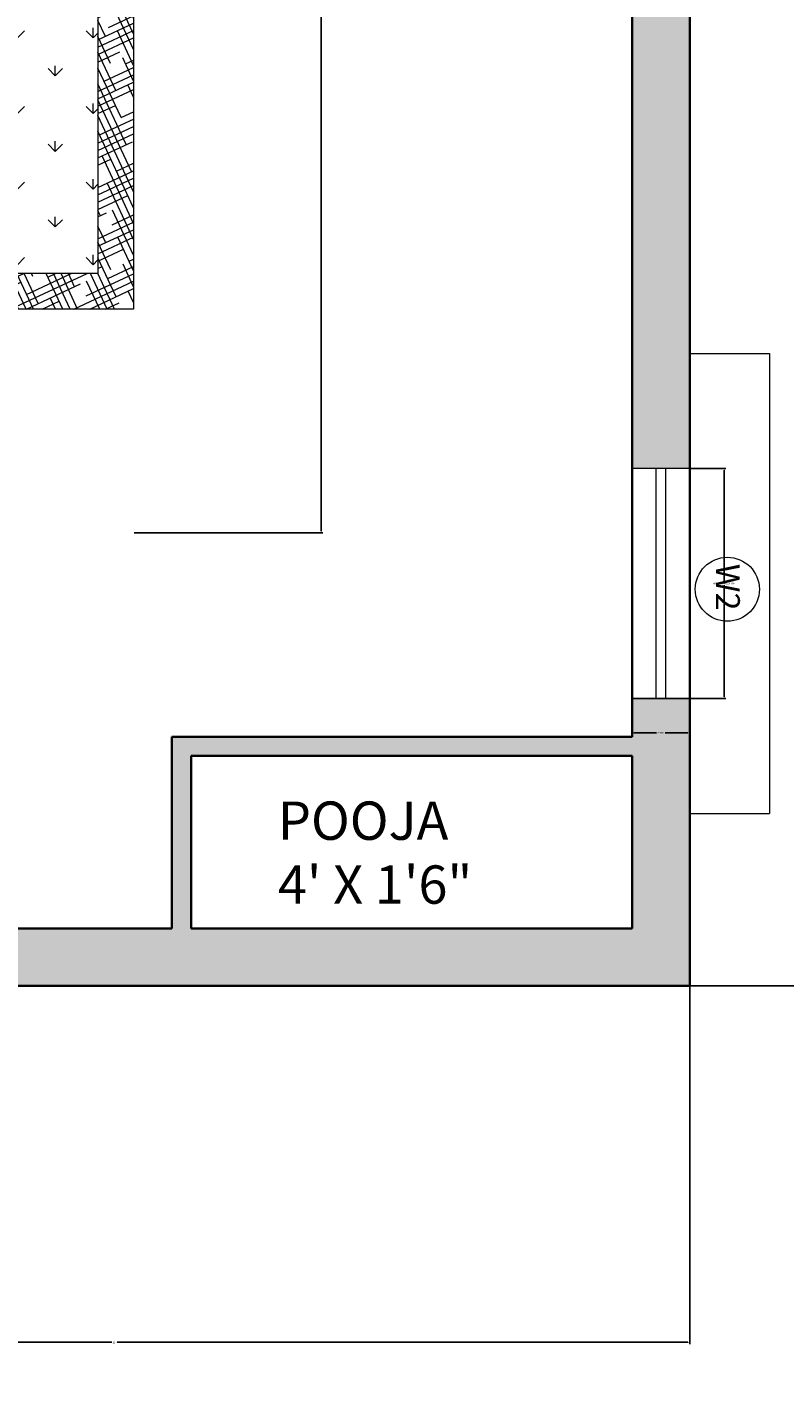
# Model space of a CAD drawing. Units: inches. Extents: x 2701 to 6846, y 811 to 2447.
# Tile 5 of 20: x 3023 to 3102, y 989 to 1130. Entities that reach past the tile are written whole.
import ezdxf

# ---------------------------------------------------------------- set-up
doc = ezdxf.new("R2010")
doc.units = ezdxf.units.IN
for name, color, linetype, lineweight in [('A-ANNO-DIMS', 2, 'Continuous', 18), ('A-ANNO-IDEN', 7, 'Continuous', 13), ('A-AREA-IDEN', 7, 'Continuous', 18), ('A-FURN', 8, 'Continuous', 13), ('A-GLAZ', 4, 'Continuous', 18), ('A-WALL', 7, 'Continuous', 35)]:
    doc.layers.add(name, color=color, linetype=linetype, lineweight=lineweight)
doc.layers.add('A-WALL-PATT', color=18, linetype='Continuous', lineweight=13, true_color=0x000000)
doc.styles.get("Standard").update_dxf_attribs({"font": 'arial.ttf'})
doc.dimstyles.get("Standard").update_dxf_attribs({"dimtxt": 0.18, "dimasz": 0.18, "dimexe": 0.18, "dimexo": 0.0625, "dimgap": 0.09, "dimtad": 0, "dimtih": 1, "dimtoh": 1, "dimdec": 4, "dimzin": 0, "dimdsep": 46, "dimtxsty": 'Standard', "dimcen": 0.09, "dimadec": 0, "dimazin": 0, "dimtfac": 1, "dimtdec": 4, "dimtofl": 0, "dimtmove": 0, "dimatfit": 3, "dimfxl": 1, "dimtolj": 1, "dimtzin": 0, "dimarcsym": 0})

# ---------------------------------------------------------------- blocks, each defined once
blk = doc.blocks.new('A$C0782773B')
for p, q in [((1027.2, 2344.2), (2528, 2344.2)), ((1508.8, 2344.2), (1508.8, 1489.7)), ((2046.4, 2344.2), (2046.4, 1489.7)), ((3223.5, 2286.1), (2888.9, 2183.3)), ((3429.1, 1617), (3223.5, 2286.1)), ((3197, 2236.1), (2938.9, 2156.8)), ((3379.1, 1643.5), (3197, 2236.1)), ((909.6, 2226.6), (909.6, 2215.4)), ((2645.6, 2226.6), (2645.6, 2215.4)), ((859.2, 2176.2), (859.2, 1545.7)), ((2696, 2176.2), (2696, 1545.7)), ((2888.9, 2183.3), (3094.6, 1514.2)), ((2938.9, 2156.8), (3121.1, 1564.2)), ((971.2, 2111.9), (971.2, 1657.7)), ((1027.2, 2097.8), (2528, 2097.8)), ((2584, 2111.9), (2584, 1657.7)), ((971.2, 2013.8), (2584, 2013.8)), ((622.9, 1770.7), (643.4, 1780.2)), ((622.9, 1750), (687.8, 1780.2)), ((622.9, 1729.3), (732.1, 1780.2)), ((622.9, 1380.2), (622.9, 1780.2)), ((622.9, 1780.2), (859.2, 1780.2)), ((627.3, 1710.7), (776.5, 1780.2)), ((636.3, 1780.2), (637.5, 1777.5)), ((657, 1780.2), (686.2, 1717.5)), ((677.6, 1780.2), (724.3, 1680.2)), ((698.3, 1780.2), (745, 1680.2)), ((703.2, 1725.4), (820.8, 1780.2)), ((719, 1780.2), (765.7, 1680.2)), ((754.2, 1749.2), (786.3, 1680.2)), ((779.1, 1740.1), (859.2, 1777.4)), ((781.1, 1780.2), (788.2, 1765)), ((801.8, 1780.2), (836.9, 1705)), ((822.5, 1780.2), (859.2, 1701.5)), ((843.2, 1780.2), (859.2, 1745.8)), ((855, 1754.8), (859.2, 1756.8)), ((2696, 1682.3), (2906.1, 1780.2)), ((2696, 1780.2), (3012.8, 1780.2)), ((2696, 1703), (2835, 1767.8)), ((2696, 1755.4), (2731, 1680.2)), ((2696, 1723.7), (2759.1, 1753.1)), ((2717.2, 1754.3), (2751.7, 1680.2)), ((2736, 1680.2), (2950.4, 1780.2)), ((2746.5, 1780.2), (2751.2, 1770.1)), ((2767.2, 1780.2), (2799.9, 1710.1)), ((2787.9, 1780.2), (2834.5, 1680.2)), ((2790.8, 1685.1), (2994.8, 1780.2)), ((2808.5, 1780.2), (2855.2, 1680.2)), ((2829.2, 1780.2), (2875.9, 1680.2)), ((2866.7, 1699.8), (3016.1, 1769.5)), ((2891.3, 1780.2), (2901.9, 1757.6)), ((2912, 1780.2), (2950.5, 1697.6)), ((2932.7, 1780.2), (2999.2, 1637.5)), ((2942.6, 1714.5), (3021.7, 1751.4)), ((2953.4, 1780.2), (3039.7, 1595.1)), ((2974, 1780.2), (3039.7, 1639.5)), ((622.9, 1720.3), (722.9, 1505.8)), ((739.5, 1680.2), (795, 1706.1)), ((783.9, 1680.2), (859.2, 1715.4)), ((2696, 1711), (2710.4, 1680.2)), ((2867.9, 1741.8), (2896.6, 1680.2)), ((3018.5, 1729.2), (3027.2, 1733.3)), ((3018.5, 1729.2), (3039.7, 1683.9)), ((622.9, 1646.6), (719.1, 1691.4)), ((622.9, 1667.2), (643.2, 1676.7)), ((622.9, 1675.9), (681.6, 1549.8)), ((622.9, 1625.9), (722.9, 1672.5)), ((652.2, 1701.6), (722.9, 1550.2)), ((722.9, 1340.4), (722.9, 1680.2)), ((722.9, 1680.2), (859.2, 1680.2)), ((802.9, 1689.1), (807, 1680.2)), ((828.2, 1680.2), (859.2, 1694.7)), ((2696, 1680.2), (2939.7, 1680.2)), ((2765.9, 1694.2), (2772.4, 1680.2)), ((2916.6, 1681.7), (2917.2, 1680.2)), ((2939.7, 1651.1), (3034.4, 1695.3)), ((2939.7, 1671.8), (2958.5, 1680.6)), ((2939.7, 1680.2), (2939.7, 1461.7)), ((2939.7, 1630.4), (3039.7, 1677.1)), ((3039.7, 1692.8), (3039.7, 1461.7)), ((622.9, 1605.2), (722.9, 1651.8)), ((622.9, 1631.5), (633, 1609.9)), ((674.9, 1608.7), (722.9, 1631.1)), ((700.9, 1641.6), (722.9, 1594.5)), ((2939.7, 1609.7), (3039.7, 1656.4)), ((2939.7, 1632.1), (3019.1, 1461.7)), ((2990.2, 1612.6), (3039.7, 1635.7)), ((3121.1, 1564.2), (3379.1, 1643.5)), ((747.4, 1598.5), (767.3, 1618.4)), ((747.4, 1598.5), (775.6, 1598.5)), ((747.4, 1598.5), (767.3, 1578.6)), ((2868.8, 1598.5), (2888.7, 1618.4)), ((2868.8, 1598.5), (2896.9, 1598.5)), ((2868.8, 1598.5), (2888.7, 1578.6)), ((2965.3, 1621.7), (3039.7, 1462)), ((3094.6, 1514.2), (3429.1, 1617)), ((622.9, 1543.1), (690.7, 1574.7)), ((622.9, 1522.4), (722.9, 1569.1)), ((2939.7, 1587.7), (2994.7, 1469.9)), ((2939.7, 1547.7), (3006, 1578.6)), ((2939.7, 1527), (3039.7, 1573.6)), ((3013.9, 1561.6), (3039.7, 1506.4)), ((622.9, 1501.7), (722.9, 1548.4)), ((622.9, 1542.8), (715.9, 1343.2)), ((646.5, 1492.1), (722.9, 1527.7)), ((647.7, 1534), (722.9, 1372.7)), ((2939.7, 1506.3), (3039.7, 1552.9)), ((2939.7, 1543.4), (2946, 1529.9)), ((2961.8, 1495.9), (3039.7, 1532.2)), ((622.9, 1498.4), (677.1, 1382.2)), ((722.4, 1506.8), (722.9, 1507)), ((853.5, 1492.5), (871.6, 1510.6)), ((853.5, 1492.5), (881.6, 1492.5)), ((853.5, 1492.5), (873.4, 1472.6)), ((915.2, 1489.7), (2640, 1489.7)), ((1068.4, 1489.7), (1085.5, 1472.6)), ((1280.5, 1489.7), (1297.7, 1472.6)), ((1492.7, 1489.7), (1509.8, 1472.6)), ((1704.8, 1489.7), (1721.9, 1472.6)), ((1916.9, 1489.7), (1934.1, 1472.6)), ((2129.1, 1489.7), (2146.2, 1472.6)), ((2341.2, 1489.7), (2358.3, 1472.6)), ((2553.3, 1489.7), (2570.5, 1472.6)), ((2762.7, 1492.5), (2782.6, 1512.3)), ((2762.7, 1492.5), (2790.8, 1492.5)), ((2762.7, 1492.5), (2782.6, 1472.6)), ((3037.7, 1510.6), (3039.7, 1511.5)), ((395.3, 1470.7), (915.7, 1263.8)), ((622.9, 1419), (722.9, 1465.6)), ((622.9, 1439.7), (662.4, 1458.1)), ((622.9, 1454.1), (628.4, 1442.2)), ((622.9, 1398.3), (722.9, 1444.9)), ((696.4, 1473.9), (722.9, 1417.1)), ((3326.7, 1461.7), (2766.7, 1461.7)), ((2977.2, 1461.7), (2977.7, 1461.9)), ((3021.6, 1461.7), (3039.7, 1470.2)), ((625.9, 1379), (722.9, 1424.2)), ((694.1, 1390.1), (722.9, 1403.5)), ((747.4, 1386.4), (767.3, 1406.3)), ((959.6, 1386.4), (979.5, 1406.3)), ((1171.7, 1386.4), (1191.6, 1406.3)), ((1383.8, 1386.4), (1403.7, 1406.3)), ((1596, 1386.4), (1615.9, 1406.3)), ((1808.1, 1386.4), (1828, 1406.3)), ((2020.2, 1386.4), (2040.1, 1406.3)), ((2232.4, 1386.4), (2252.3, 1406.3)), ((2444.5, 1386.4), (2464.4, 1406.3)), ((2656.6, 1386.4), (2676.5, 1406.3)), ((2710.7, 1349.7), (2710.7, 1405.7)), ((747.4, 1386.4), (775.6, 1386.4)), ((747.4, 1386.4), (767.3, 1366.5)), ((959.6, 1386.4), (987.7, 1386.4)), ((959.6, 1386.4), (979.5, 1366.5)), ((1171.7, 1386.4), (1199.8, 1386.4)), ((1171.7, 1386.4), (1191.6, 1366.5)), ((1383.8, 1386.4), (1412, 1386.4)), ((1383.8, 1386.4), (1403.7, 1366.5)), ((1596, 1386.4), (1624.1, 1386.4)), ((1596, 1386.4), (1615.9, 1366.5)), ((1808.1, 1386.4), (1836.2, 1386.4)), ((1808.1, 1386.4), (1828, 1366.5)), ((2020.2, 1386.4), (2048.4, 1386.4)), ((2020.2, 1386.4), (2040.1, 1366.5)), ((2232.4, 1386.4), (2260.5, 1386.4)), ((2232.4, 1386.4), (2252.3, 1366.5)), ((2444.5, 1386.4), (2472.6, 1386.4)), ((2444.5, 1386.4), (2464.4, 1366.5)), ((2656.6, 1386.4), (2684.8, 1386.4)), ((2656.6, 1386.4), (2676.5, 1366.5)), ((413.6, 1342.9), (770.2, 1201.1)), ((697.7, 1350.4), (709.9, 1356.1)), ((721.7, 1340.9), (722.9, 1341.5)), ((2710.7, 1349.7), (2710.7, 733.3)), ((3262.5, 1349.7), (2878.7, 1349.7)), ((3164.3, 1349.7), (3164.3, 789.3)), ((11.5, 960), (148, 1303.4)), ((297.8, 785.9), (504.9, 1306.6)), ((859.4, 1286.2), (873.4, 1300.2)), ((1065.6, 1280.3), (1085.5, 1300.2)), ((1277.8, 1280.3), (1297.7, 1300.2)), ((1489.9, 1280.3), (1509.8, 1300.2)), ((1702, 1280.3), (1721.9, 1300.2)), ((1914.2, 1280.3), (1934.1, 1300.2)), ((2126.3, 1280.3), (2146.2, 1300.2)), ((2338.4, 1280.3), (2358.3, 1300.2)), ((2550.6, 1280.3), (2570.5, 1300.2)), ((3248.3, 1293.7), (3248.3, 924.1)), ((3494.7, 1293.7), (3494.7, 924.1)), ((874.1, 1280.3), (881.6, 1280.3)), ((1065.6, 1280.3), (1093.8, 1280.3)), ((1065.6, 1280.3), (1085.5, 1260.4)), ((1277.8, 1280.3), (1305.9, 1280.3)), ((1277.8, 1280.3), (1297.7, 1260.4)), ((1489.9, 1280.3), (1518, 1280.3)), ((1489.9, 1280.3), (1509.8, 1260.4)), ((1702, 1280.3), (1730.2, 1280.3)), ((1702, 1280.3), (1721.9, 1260.4)), ((1914.2, 1280.3), (1942.3, 1280.3)), ((1914.2, 1280.3), (1934.1, 1260.4)), ((2126.3, 1280.3), (2154.4, 1280.3)), ((2126.3, 1280.3), (2146.2, 1260.4)), ((2338.4, 1280.3), (2366.6, 1280.3)), ((2338.4, 1280.3), (2358.3, 1260.4)), ((2550.6, 1280.3), (2578.7, 1280.3)), ((2550.6, 1280.3), (2570.5, 1260.4)), ((240.4, 868.9), (377, 1212.4)), ((719.3, 618.3), (947, 1191)), ((959.6, 1174.3), (979.5, 1194.1)), ((1171.7, 1174.3), (1191.6, 1194.1)), ((1383.8, 1174.3), (1403.7, 1194.1)), ((1596, 1174.3), (1615.9, 1194.1)), ((1808.1, 1174.3), (1828, 1194.1)), ((2020.2, 1174.3), (2040.1, 1194.1)), ((2232.4, 1174.3), (2252.3, 1194.1)), ((2444.5, 1174.3), (2464.4, 1194.1)), ((2656.6, 1174.3), (2676.5, 1194.1)), ((959.6, 1174.3), (987.7, 1174.3)), ((959.6, 1174.3), (979.5, 1154.4)), ((1171.7, 1174.3), (1199.8, 1174.3)), ((1171.7, 1174.3), (1191.6, 1154.4)), ((1383.8, 1174.3), (1412, 1174.3)), ((1383.8, 1174.3), (1403.7, 1154.4)), ((1596, 1174.3), (1624.1, 1174.3)), ((1596, 1174.3), (1615.9, 1154.4)), ((1808.1, 1174.3), (1836.2, 1174.3)), ((1808.1, 1174.3), (1828, 1154.4)), ((2020.2, 1174.3), (2048.4, 1174.3)), ((2020.2, 1174.3), (2040.1, 1154.4)), ((2232.4, 1174.3), (2260.5, 1174.3)), ((2232.4, 1174.3), (2252.3, 1154.4)), ((2444.5, 1174.3), (2472.6, 1174.3)), ((2444.5, 1174.3), (2464.4, 1154.4)), ((2656.6, 1174.3), (2684.8, 1174.3)), ((2656.6, 1174.3), (2676.5, 1154.4)), ((1358.2, 528.2), (1358.2, 1102.6)), ((1358.2, 1102.6), (2266.7, 1102.6)), ((2266.7, 1102.6), (2266.7, 528.2)), ((1065.6, 1068.2), (1085.5, 1088.1)), ((1065.6, 1068.2), (1093.8, 1068.2)), ((1065.6, 1068.2), (1085.5, 1048.3)), ((1277.8, 1068.2), (1297.7, 1088.1)), ((1277.8, 1068.2), (1305.9, 1068.2)), ((1277.8, 1068.2), (1297.7, 1048.3)), ((2338.4, 1068.2), (2358.3, 1088.1)), ((2338.4, 1068.2), (2366.6, 1068.2)), ((2338.4, 1068.2), (2358.3, 1048.3)), ((2550.6, 1068.2), (2570.5, 1088.1)), ((2550.6, 1068.2), (2578.7, 1068.2)), ((2550.6, 1068.2), (2570.5, 1048.3)), ((1408.2, 578.2), (1408.2, 1052.6)), ((1408.2, 1052.6), (2216.7, 1052.6)), ((1408.2, 1031.9), (1644.7, 847.1)), ((1437.7, 1052.6), (1999.3, 613.9)), ((1510.8, 1052.6), (2118.1, 578.2)), ((1674, 1052.6), (1887.9, 885.5)), ((1681.3, 1052.6), (2216.7, 634.3)), ((1738, 1027.4), (2092.6, 750.4)), ((1837.3, 1052.6), (1926.1, 983.2)), ((1925, 1052.6), (2216.7, 824.7)), ((2000.5, 1052.6), (2216.7, 883.7)), ((2029.7, 1052.6), (2097.2, 999.9)), ((2163.7, 1052.6), (2215.4, 1012.3)), ((2168.6, 1052.6), (2216.7, 1015)), ((2216.7, 1052.6), (2216.7, 578.2)), ((1408.2, 1005.3), (1598.7, 856.4)), ((959.6, 962.1), (979.5, 982)), ((959.6, 962.1), (987.7, 962.1)), ((959.6, 962.1), (979.5, 942.2)), ((1171.7, 962.1), (1191.6, 982)), ((1171.7, 962.1), (1199.8, 962.1)), ((1171.7, 962.1), (1191.6, 942.2)), ((2136.2, 969.5), (2216.7, 906.5)), ((2444.5, 962.1), (2464.4, 982)), ((2444.5, 962.1), (2472.6, 962.1)), ((2444.5, 962.1), (2464.4, 942.2)), ((2656.6, 962.1), (2676.5, 982)), ((2656.6, 962.1), (2684.8, 962.1)), ((2656.6, 962.1), (2676.5, 942.2)), ((853.5, 856.1), (873.4, 876)), ((1065.6, 856.1), (1085.5, 876)), ((1277.8, 856.1), (1297.7, 876)), ((1408.2, 885.3), (1646.9, 698.8)), ((1408.2, 877.7), (1560.4, 758.8)), ((2338.4, 856.1), (2358.3, 876)), ((2550.6, 856.1), (2570.5, 876)), ((853.5, 856.1), (881.6, 856.1)), ((853.5, 856.1), (873.4, 836.2)), ((1065.6, 856.1), (1093.8, 856.1)), ((1065.6, 856.1), (1085.5, 836.2)), ((1277.8, 856.1), (1305.9, 856.1)), ((1277.8, 856.1), (1297.7, 836.2)), ((2091.6, 853.9), (2216.7, 756.2)), ((2338.4, 856.1), (2366.6, 856.1)), ((2338.4, 856.1), (2358.3, 836.2)), ((2550.6, 856.1), (2578.7, 856.1)), ((2550.6, 856.1), (2570.5, 836.2)), ((206.6, 822.1), (563.2, 680.3)), ((959.6, 750), (979.5, 769.9)), ((1171.7, 750), (1191.6, 769.9)), ((1408.2, 778.7), (1640.1, 597.6)), ((1733.4, 777.9), (1989, 578.2)), ((2006.1, 793.2), (2216.7, 628.6)), ((2444.5, 750), (2464.4, 769.9)), ((2656.6, 750), (2676.5, 769.9)), ((3262.5, 789.3), (2878.7, 789.3)), ((105.5, 741.8), (625.9, 534.9)), ((764.8, 732.7), (767.3, 730.1)), ((771.7, 750), (775.6, 750)), ((959.6, 750), (987.7, 750)), ((959.6, 750), (979.5, 730.1)), ((1171.7, 750), (1199.8, 750)), ((1171.7, 750), (1191.6, 730.1)), ((1408.2, 750.2), (1628.4, 578.2)), ((1764.2, 727.1), (1954.8, 578.2)), ((2131.6, 719.9), (2216.7, 653.4)), ((2444.5, 750), (2472.6, 750)), ((2444.5, 750), (2464.4, 730.1)), ((2656.6, 750), (2684.8, 750)), ((2656.6, 750), (2676.5, 730.1)), ((853.5, 643.9), (873.4, 663.8)), ((1065.6, 643.9), (1085.5, 663.8)), ((1277.8, 643.9), (1297.7, 663.8)), ((1678.6, 666.4), (1791.6, 578.2)), ((2338.4, 643.9), (2358.3, 663.8)), ((2550.6, 643.9), (2570.5, 663.8)), ((2762.7, 643.9), (2782.6, 663.8)), ((3326.7, 677.3), (2766.7, 677.3)), ((2939.7, 658.1), (2981, 677.3)), ((2939.7, 637.4), (3025.4, 677.3)), ((2939.7, 677.3), (2939.7, 567.7)), ((2939.7, 616.7), (3039.7, 663.3)), ((2950.4, 677.3), (2971.8, 631.6)), ((2971.1, 677.3), (3020.4, 571.6)), ((2991.8, 677.3), (3039.7, 574.7)), ((3012.5, 677.3), (3039.7, 619.1)), ((3039.7, 677.3), (3039.7, 567.7)), ((719.3, 618.3), (698.6, 566.2)), ((722.9, 100), (722.9, 627.2)), ((853.5, 643.9), (881.6, 643.9)), ((853.5, 643.9), (873.4, 624)), ((1065.6, 643.9), (1093.8, 643.9)), ((1065.6, 643.9), (1085.5, 624)), ((1277.8, 643.9), (1305.9, 643.9)), ((1277.8, 643.9), (1297.7, 624)), ((2338.4, 643.9), (2366.6, 643.9)), ((2338.4, 643.9), (2358.3, 624)), ((2550.6, 643.9), (2578.7, 643.9)), ((2550.6, 643.9), (2570.5, 624)), ((2762.7, 643.9), (2790.8, 643.9)), ((2762.7, 643.9), (2782.6, 624)), ((2939.7, 611.7), (2960.2, 567.7)), ((2962.7, 606.7), (3039.7, 642.6)), ((3038.6, 621.4), (3039.7, 621.9)), ((697.8, 564.3), (722.9, 576)), ((701.9, 574.6), (722.9, 529.8)), ((722.1, 575.7), (722.9, 574.1)), ((2216.7, 578.2), (1408.2, 578.2)), ((1436.7, 600.4), (1465.1, 578.2)), ((1530.9, 599.1), (1557.7, 578.2)), ((2967.7, 567.7), (2978.5, 572.7)), ((3012, 567.7), (3039.7, 580.6)), ((622.9, 508.7), (722.9, 555.3)), ((622.9, 0), (622.9, 536.1)), ((622.9, 488), (722.9, 534.6)), ((622.9, 529.4), (630.9, 533.1)), ((676.8, 539.8), (702.9, 483.9)), ((691.3, 553.2), (722.9, 485.4)), ((747.4, 537.9), (767.3, 557.8)), ((747.4, 537.9), (775.6, 537.9)), ((747.4, 537.9), (767.3, 518)), ((959.6, 537.9), (979.5, 557.8)), ((959.6, 537.9), (987.7, 537.9)), ((959.6, 537.9), (979.5, 518)), ((1171.7, 537.9), (1191.6, 557.8)), ((1171.7, 537.9), (1199.8, 537.9)), ((1171.7, 537.9), (1191.6, 518)), ((2444.5, 537.9), (2464.4, 557.8)), ((2444.5, 537.9), (2472.6, 537.9)), ((2444.5, 537.9), (2464.4, 518)), ((2656.6, 537.9), (2676.5, 557.8)), ((2656.6, 537.9), (2684.8, 537.9)), ((2656.6, 537.9), (2676.5, 518)), ((2868.8, 537.9), (2873.3, 542.4)), ((2868.8, 537.9), (2873.3, 537.9)), ((2868.8, 537.9), (2873.3, 533.3)), ((2873.3, 567.7), (3323.3, 567.7)), ((2873.3, 117.7), (2873.3, 567.7)), ((3323.3, 567.7), (3323.3, 117.7)), ((622.9, 522.4), (722.9, 307.9)), ((694.9, 500.9), (722.9, 513.9)), ((2266.7, 528.2), (1358.2, 528.2)), ((1393.5, 528.2), (1403.7, 518)), ((1605.7, 528.2), (1615.9, 518)), ((1817.8, 528.2), (1828, 518)), ((2029.9, 528.2), (2040.1, 518)), ((2242.1, 528.2), (2252.3, 518)), ((3098.3, 156.5), (3098.3, 526.4)), ((622.9, 478), (698.3, 316.3)), ((622.9, 425.9), (710.8, 466.9)), ((668.9, 468.1), (722.9, 352.3)), ((622.9, 446.6), (634.9, 452.2)), ((622.9, 405.3), (722.9, 451.9)), ((622.9, 433.6), (649.6, 376.3)), ((622.9, 384.6), (722.9, 431.2)), ((853.5, 431.8), (873.4, 451.7)), ((853.5, 431.8), (881.6, 431.8)), ((853.5, 431.8), (873.4, 411.9)), ((1065.6, 431.8), (1085.5, 451.7)), ((1065.6, 431.8), (1093.8, 431.8)), ((1065.6, 431.8), (1085.5, 411.9)), ((1277.8, 431.8), (1297.7, 451.7)), ((1277.8, 431.8), (1305.9, 431.8)), ((1277.8, 431.8), (1297.7, 411.9)), ((1489.9, 431.8), (1509.8, 451.7)), ((1489.9, 431.8), (1518, 431.8)), ((1489.9, 431.8), (1509.8, 411.9)), ((1702, 431.8), (1721.9, 451.7)), ((1702, 431.8), (1730.2, 431.8)), ((1702, 431.8), (1721.9, 411.9)), ((1914.2, 431.8), (1934.1, 451.7)), ((1914.2, 431.8), (1942.3, 431.8)), ((1914.2, 431.8), (1934.1, 411.9)), ((2126.3, 431.8), (2146.2, 451.7)), ((2126.3, 431.8), (2154.4, 431.8)), ((2126.3, 431.8), (2146.2, 411.9)), ((2338.4, 431.8), (2358.3, 451.7)), ((2338.4, 431.8), (2366.6, 431.8)), ((2338.4, 431.8), (2358.3, 411.9)), ((2550.6, 431.8), (2570.5, 451.7)), ((2550.6, 431.8), (2578.7, 431.8)), ((2550.6, 431.8), (2570.5, 411.9)), ((2762.7, 431.8), (2782.6, 451.7)), ((2762.7, 431.8), (2790.8, 431.8)), ((2762.7, 431.8), (2782.6, 411.9)), ((666.6, 384.3), (722.9, 410.5)), ((717.6, 408), (722.9, 396.7)), ((622.9, 322.5), (682.4, 350.3)), ((622.9, 301.8), (722.9, 348.4)), ((622.9, 344.9), (722.9, 130.5)), ((747.4, 325.7), (767.3, 345.6)), ((959.6, 325.7), (979.5, 345.6)), ((1171.7, 325.7), (1191.6, 345.6)), ((1383.8, 325.7), (1403.7, 345.6)), ((1596, 325.7), (1615.9, 345.6)), ((1808.1, 325.7), (1828, 345.6)), ((2020.2, 325.7), (2040.1, 345.6)), ((2232.4, 325.7), (2252.3, 345.6)), ((2444.5, 325.7), (2464.4, 345.6)), ((2656.6, 325.7), (2676.5, 345.6)), ((2914.5, 342.7), (3284.1, 342.7)), ((622.9, 281.1), (722.9, 327.8)), ((638.2, 267.6), (722.9, 307.1)), ((747.4, 325.7), (775.6, 325.7)), ((747.4, 325.7), (767.3, 305.8)), ((959.6, 325.7), (987.7, 325.7)), ((959.6, 325.7), (979.5, 305.8)), ((1171.7, 325.7), (1199.8, 325.7)), ((1171.7, 325.7), (1191.6, 305.8)), ((1383.8, 325.7), (1412, 325.7)), ((1383.8, 325.7), (1403.7, 305.8)), ((1596, 325.7), (1624.1, 325.7)), ((1596, 325.7), (1615.9, 305.8)), ((1808.1, 325.7), (1836.2, 325.7)), ((1808.1, 325.7), (1828, 305.8)), ((2020.2, 325.7), (2048.4, 325.7)), ((2020.2, 325.7), (2040.1, 305.8)), ((2232.4, 325.7), (2260.5, 325.7)), ((2232.4, 325.7), (2252.3, 305.8)), ((2444.5, 325.7), (2472.6, 325.7)), ((2444.5, 325.7), (2464.4, 305.8)), ((2656.6, 325.7), (2684.8, 325.7)), ((2656.6, 325.7), (2676.5, 305.8)), ((2868.8, 325.7), (2873.3, 330.3)), ((2868.8, 325.7), (2873.3, 325.7)), ((2868.8, 325.7), (2873.3, 321.2)), ((622.9, 300.5), (693.7, 148.6)), ((664.3, 300.4), (722.9, 174.8)), ((714.1, 282.3), (722.9, 286.4)), ((622.9, 256.2), (645, 208.7)), ((622.9, 198.4), (722.9, 245)), ((622.9, 219.1), (654.1, 233.6)), ((713, 240.4), (722.9, 219.2)), ((853.5, 219.7), (873.4, 239.6)), ((1065.6, 219.7), (1085.5, 239.6)), ((1277.8, 219.7), (1297.7, 239.6)), ((1489.9, 219.7), (1509.8, 239.6)), ((1702, 219.7), (1721.9, 239.6)), ((1914.2, 219.7), (1934.1, 239.6)), ((2126.3, 219.7), (2146.2, 239.6)), ((2338.4, 219.7), (2358.3, 239.6)), ((2550.6, 219.7), (2570.5, 239.6)), ((2762.7, 219.7), (2782.6, 239.6)), ((622.9, 177.7), (722.9, 224.3)), ((622.9, 157), (722.9, 203.6)), ((853.5, 219.7), (881.6, 219.7)), ((853.5, 219.7), (873.4, 199.8)), ((1065.6, 219.7), (1093.8, 219.7)), ((1065.6, 219.7), (1085.5, 199.8)), ((1277.8, 219.7), (1305.9, 219.7)), ((1277.8, 219.7), (1297.7, 199.8)), ((1489.9, 219.7), (1518, 219.7)), ((1489.9, 219.7), (1509.8, 199.8)), ((1702, 219.7), (1730.2, 219.7)), ((1702, 219.7), (1721.9, 199.8)), ((1914.2, 219.7), (1942.3, 219.7)), ((1914.2, 219.7), (1934.1, 199.8)), ((2126.3, 219.7), (2154.4, 219.7)), ((2126.3, 219.7), (2146.2, 199.8)), ((2338.4, 219.7), (2366.6, 219.7)), ((2338.4, 219.7), (2358.3, 199.8)), ((2550.6, 219.7), (2578.7, 219.7)), ((2550.6, 219.7), (2570.5, 199.8)), ((2762.7, 219.7), (2790.8, 219.7)), ((2762.7, 219.7), (2782.6, 199.8)), ((622.9, 167.4), (700.9, 0)), ((685.8, 165.6), (722.9, 182.9)), ((622.9, 94.9), (701.6, 131.7)), ((622.9, 123.1), (680.3, 0)), ((622.9, 74.2), (722.9, 120.9)), ((622.9, 115.6), (625.7, 116.9)), ((659.7, 132.8), (721.6, 0)), ((747.4, 113.6), (767.3, 133.5)), ((959.6, 113.6), (979.5, 133.5)), ((1171.7, 113.6), (1191.6, 133.5)), ((1383.8, 113.6), (1403.7, 133.5)), ((1596, 113.6), (1615.9, 133.5)), ((1808.1, 113.6), (1828, 133.5)), ((2020.2, 113.6), (2040.1, 133.5)), ((2232.4, 113.6), (2252.3, 133.5)), ((2444.5, 113.6), (2464.4, 133.5)), ((2656.6, 113.6), (2676.5, 133.5)), ((2745, 8.7), (2978.7, 117.7)), ((2820.9, 23.4), (3023, 117.7)), ((2868.8, 113.6), (2873.3, 118.1)), ((3323.3, 117.7), (2873.3, 117.7)), ((2939.7, 117.7), (2939.7, 100)), ((2983.9, 117.7), (3006.7, 68.7)), ((3004.5, 117.7), (3039.7, 42.3)), ((3025.2, 117.7), (3039.7, 86.7)), ((3039.7, 117.7), (3039.7, 0)), ((622.9, 53.5), (722.9, 100.2)), ((622.9, 78.7), (640.4, 41)), ((657.4, 49), (766.8, 100)), ((2939.7, 100), (722.9, 100)), ((733.3, 63.7), (811.2, 100)), ((737.1, 100), (742.4, 88.6)), ((747.4, 113.6), (775.6, 113.6)), ((747.4, 113.6), (761, 100)), ((757.8, 100), (791.1, 28.5)), ((778.4, 100), (825.1, 0)), ((799.1, 100), (845.8, 0)), ((809.2, 78.4), (855.6, 100)), ((819.8, 100), (866.5, 0)), ((863, 0), (1052.8, 88.5)), ((881.9, 100), (893, 76.1)), ((885.1, 93.1), (899.9, 100)), ((902.6, 100), (941.7, 16)), ((907.3, 0), (1121.8, 100)), ((923.3, 100), (969.9, 0)), ((943.9, 100), (990.6, 0)), ((951.7, 0), (1166.1, 100)), ((959.6, 113.6), (987.7, 113.6)), ((959.6, 113.6), (973.2, 100)), ((964.6, 100), (1011.3, 0)), ((1008.6, 5.8), (1210.5, 100)), ((1026.7, 100), (1043.7, 63.6)), ((1047.4, 100), (1092.4, 3.5)), ((1068.1, 100), (1114.7, 0)), ((1084.4, 20.5), (1254.9, 100)), ((1088.8, 100), (1135.4, 0)), ((1111.7, 95.3), (1156.1, 0)), ((1160.3, 35.2), (1299.2, 100)), ((1171.5, 100), (1194.3, 51.1)), ((1171.7, 113.6), (1199.8, 113.6)), ((1171.7, 113.6), (1185.3, 100)), ((1192.2, 100), (1238.8, 0)), ((1212.9, 100), (1259.5, 0)), ((1233.6, 100), (1280.2, 0)), ((1236.2, 49.9), (1343.6, 100)), ((1262.3, 82.8), (1300.9, 0)), ((1295.7, 100), (1296.3, 98.6)), ((1312.1, 64.6), (1388, 100)), ((1316.3, 100), (1345, 38.6)), ((1337, 100), (1383.7, 0)), ((1357.7, 100), (1404.3, 0)), ((1378.4, 100), (1425, 0)), ((1383.8, 113.6), (1412, 113.6)), ((1383.8, 113.6), (1397.4, 100)), ((1388, 79.3), (1432.3, 100)), ((1439.7, 0), (1631.6, 89.5)), ((1440.5, 100), (1446.9, 86.1)), ((1461.2, 100), (1495.6, 26.1)), ((1463.9, 94), (1476.7, 100)), ((1481.8, 100), (1528.5, 0)), ((1484.1, 0), (1698.5, 100)), ((1502.5, 100), (1549.2, 0)), ((1523.2, 100), (1569.9, 0)), ((1528.5, 0), (1742.9, 100)), ((1585.3, 100), (1597.6, 73.6)), ((1587.4, 6.8), (1787.3, 100)), ((1596, 113.6), (1624.1, 113.6)), ((1596, 113.6), (1609.6, 100)), ((1606, 100), (1646.3, 13.6)), ((1626.7, 100), (1673.3, 0)), ((1647.4, 100), (1694, 0)), ((1663.3, 21.5), (1831.6, 100)), ((1668, 100), (1714.7, 0)), ((1730.1, 100), (1748.2, 61.1)), ((1739.2, 36.2), (1876, 100)), ((1750.8, 100), (1796.9, 1.1)), ((1771.5, 100), (1818.1, 0)), ((1792.2, 100), (1838.8, 0)), ((1808.1, 113.6), (1836.2, 113.6)), ((1808.1, 113.6), (1821.7, 100)), ((1815.1, 50.9), (1920.4, 100)), ((1816.2, 92.8), (1859.5, 0)), ((1874.9, 100), (1898.9, 48.6)), ((1891, 65.6), (1964.7, 100)), ((1895.6, 100), (1942.2, 0)), ((1916.3, 100), (1962.9, 0)), ((1937, 100), (1983.6, 0)), ((1966.9, 80.3), (2009.1, 100)), ((1966.9, 80.3), (2004.3, 0)), ((1999.1, 100), (2000.8, 96.2)), ((2016.5, 0), (2210.4, 90.4)), ((2019.7, 100), (2049.5, 36.1)), ((2020.2, 113.6), (2048.4, 113.6)), ((2020.2, 113.6), (2033.8, 100)), ((2040.4, 100), (2087.1, 0)), ((2042.8, 95), (2053.5, 100)), ((2060.8, 0), (2275.3, 100)), ((2061.1, 100), (2107.8, 0)), ((2081.8, 100), (2128.4, 0)), ((2105.2, 0), (2319.7, 100)), ((2143.9, 100), (2151.5, 83.6)), ((2164.6, 100), (2200.2, 23.6)), ((2166.2, 7.8), (2364, 100)), ((2185.2, 100), (2231.9, 0)), ((2205.9, 100), (2252.6, 0)), ((2226.6, 100), (2273.3, 0)), ((2232.4, 113.6), (2260.5, 113.6)), ((2232.4, 113.6), (2246, 100)), ((2242.1, 22.5), (2408.4, 100)), ((2288.7, 100), (2302.1, 71.1)), ((2309.4, 100), (2350.8, 11.1)), ((2318, 37.2), (2452.8, 100)), ((2330.1, 100), (2376.7, 0)), ((2350.8, 100), (2397.4, 0)), ((2371.4, 100), (2418.1, 0)), ((2393.9, 51.9), (2497.1, 100)), ((2433.5, 100), (2452.8, 58.6)), ((2444.5, 113.6), (2472.6, 113.6)), ((2444.5, 113.6), (2458.1, 100)), ((2454.2, 100), (2500.8, 0)), ((2469.8, 66.6), (2541.5, 100)), ((2474.9, 100), (2521.5, 0)), ((2495.6, 100), (2542.2, 0)), ((2520.8, 90.3), (2562.9, 0)), ((2545.7, 81.3), (2585.9, 100)), ((2548.9, 0), (2713.3, 76.7)), ((2578.3, 100), (2603.4, 46.1)), ((2593.2, 0), (2789.2, 91.4)), ((2599, 100), (2645.6, 0)), ((2619.7, 100), (2666.3, 0)), ((2621.6, 96), (2630.2, 100)), ((2637.6, 0), (2852.1, 100)), ((2640.4, 100), (2687, 0)), ((2656.6, 113.6), (2684.8, 113.6)), ((2656.6, 113.6), (2670.2, 100)), ((2671.4, 77.8), (2707.7, 0)), ((2682, 0), (2896.4, 100)), ((2702.5, 100), (2705.4, 93.7)), ((2723.1, 100), (2754.1, 33.6)), ((2743.8, 100), (2790.5, 0)), ((2764.5, 100), (2811.2, 0)), ((2785.2, 100), (2831.8, 0)), ((2847.3, 100), (2856.1, 81.2)), ((2868, 100), (2904.7, 21.1)), ((2868.8, 113.6), (2896.9, 113.6)), ((2868.8, 113.6), (2882.4, 100)), ((2888.7, 100), (2935.3, 0)), ((2896.8, 38.1), (3039.7, 104.7)), ((2909.3, 100), (2956, 0)), ((2930, 100), (2976.7, 0)), ((2972.7, 52.8), (3039.7, 84.1)), ((708.4, 72.7), (742.3, 0)), ((729.9, 0), (825.1, 44.4)), ((774.2, 0), (901, 59.1)), ((818.6, 0), (976.9, 73.8)), ((859, 60.2), (887.1, 0)), ((1009.7, 47.7), (1032, 0)), ((1306.6, 0), (1403.9, 45.4)), ((1351, 0), (1479.8, 60.1)), ((1395.4, 0), (1555.7, 74.8)), ((1413, 70.3), (1445.7, 0)), ((1563.6, 57.8), (1590.5, 0)), ((1714.3, 45.3), (1735.4, 0)), ((1883.4, 0), (1982.7, 46.3)), ((1927.7, 0), (2058.6, 61)), ((1972.1, 0), (2134.5, 75.7)), ((2117.5, 67.8), (2149.1, 0)), ((2268.2, 55.3), (2293.9, 0)), ((2418.8, 42.8), (2438.8, 0)), ((2460.1, 0), (2561.5, 47.3)), ((2504.5, 0), (2637.4, 62)), ((2822.1, 65.3), (2852.5, 0)), ((2972.7, 52.8), (2997.3, 0)), ((641.1, 0), (673.3, 15)), ((685.5, 0), (749.2, 29.7)), ((757.1, 12.7), (763, 0)), ((907.7, 0.2), (907.8, 0)), ((1160.3, 35.2), (1176.8, 0)), ((1173.5, 0), (1176.2, 1.2)), ((1217.9, 0), (1252.1, 15.9)), ((1262.3, 0), (1328, 30.7)), ((1311, 22.7), (1321.6, 0)), ((1461.6, 10.2), (1466.4, 0)), ((1750.3, 0), (1755, 2.2)), ((1794.6, 0), (1830.9, 16.9)), ((1839, 0), (1906.8, 31.6)), ((1864.9, 32.8), (1880.2, 0)), ((2015.6, 20.3), (2025, 0)), ((2166.2, 7.8), (2169.8, 0)), ((2327, 0), (2333.8, 3.2)), ((2371.4, 0), (2409.7, 17.9)), ((2415.8, 0), (2485.6, 32.6)), ((2569.5, 30.3), (2583.6, 0)), ((2720.1, 17.8), (2728.4, 0)), ((2870.8, 5.3), (2873.2, 0)), ((2903.8, 0), (2912.7, 4.1)), ((2948.2, 0), (2988.6, 18.8)), ((2992.5, 0), (3039.7, 22)), ((3036.9, 0), (3039.7, 1.3)), ((3039.7, 0), (622.9, 0))]:
    blk.add_line(p, q)
for radius in [150, 70]:
    blk.add_circle((3098.3, 342.7), radius)
for centre, radius, start, end in [((1027.2, 2176.2), 168, 90, 180), ((1027.2, 2226.6), 117.6, 90, 180), ((2528, 2176.2), 168, 0, 90), ((2528, 2226.6), 117.6, 0, 90), ((1027.2, 2215.4), 117.6, 180, 270), ((2528, 2215.4), 117.6, 270, 0), ((915.2, 1657.7), 56, 180, 0), ((2640, 1657.7), 56, 180, 0), ((915.2, 1545.7), 56, 180, 270), ((2640, 1545.7), 56, 270, 0), ((384.7, 1219.9), 251, 87.5849, 160.561), ((344, 1235.6), 207.4, 93.9069, 160.9015), ((2766.7, 1405.7), 56, 90, 180), ((2878.7, 1405.7), 56, 90, 270), ((3326.7, 1293.7), 168, 0, 90), ((187.9, 1297.6), 207.4, 335.733, 42.7275), ((3365.9, 1293.7), 117.6, 90, 180), ((3377.1, 1293.7), 117.6, 0, 90), ((790.9, 1253.1), 56, 248.3172, 68.3172), ((895, 1211.7), 56, 338.3172, 68.3172), ((167.6, 897.9), 168, 158.3172, 248.3172), ((120.8, 916.5), 117.6, 158.3172, 248.3172), ((3455.5, 914.8), 207.4, 177.4158, 244.4103), ((3243.9, 914.3), 251, 289.2676, 2.2438), ((3287.6, 914.8), 207.4, 295.5897, 2.5842), ((131.2, 912.4), 117.6, 248.3172, 338.3172), ((2878.7, 733.3), 56, 90, 270), ((2766.7, 733.3), 56, 180, 270), ((542.5, 628.3), 56, 248.3172, 68.3172), ((646.6, 586.9), 56, 248.3172, 338.3172)]:
    blk.add_arc(centre, radius, start, end)
blk = doc.blocks.new('WIN-W2-24IN')
for p, q in [((24, 6), (0, 6)), ((24, 6), (0, 6)), ((0, 0), (0, 6)), ((24, 6), (24, 6)), ((24, 6), (24, 0)), ((24, 3.5), (0, 3.5)), ((24, 2.5), (0, 2.5)), ((24, 0), (0, 0))]:
    blk.add_line(p, q)
blk = doc.blocks.new('*D35')
at = {"layer": 'A-ANNO-DIMS', "color": 0, "lineweight": -2, "transparency": 16777216}
for p, q in [((3092.03, 1084.05), (3095.75, 1084.05)), ((3095.57, 1083.87), (3095.57, 1072.23)), ((3095.57, 1060.23), (3095.57, 1071.87)), ((3092.03, 1060.05), (3095.75, 1060.05))]:
    blk.add_line(p, q, dxfattribs=at)
at = {"layer": 'A-ANNO-DIMS', "color": 0, "transparency": 16777216}
for points in [[(3095.54, 1083.87), (3095.6, 1083.87), (3095.57, 1084.05)], [(3095.54, 1060.23), (3095.6, 1060.23), (3095.57, 1060.05)]]:
    blk.add_solid(points, dxfattribs=at)
at = {"layer": 'Defpoints', "color": 0, "transparency": 16777216}
for p in [(3091.97, 1084.05), (3091.97, 1060.05), (3095.57, 1060.05)]:
    blk.add_point(p, dxfattribs=at)
at = {"layer": 'A-ANNO-DIMS', "color": 0, "transparency": 16777216, "insert": (3095.57, 1072.05), "char_height": 0.18, "attachment_point": 5}
blk.add_mtext('\\A1;WINDOW W2 24 TYP.', dxfattribs=at)
blk = doc.blocks.new('*D36')
at = {"layer": 'A-ANNO-DIMS', "color": 0, "lineweight": -2, "transparency": 16777216}
for p, q in [((3085.97, 1059.99), (3085.97, 1056.27)), ((3091.97, 1059.99), (3091.97, 1056.27)), ((3086.15, 1056.45), (3088.51, 1056.45)), ((3091.79, 1056.45), (3089.43, 1056.45))]:
    blk.add_line(p, q, dxfattribs=at)
at = {"layer": 'A-ANNO-DIMS', "color": 0, "transparency": 16777216}
for points in [[(3086.15, 1056.48), (3086.15, 1056.42), (3085.97, 1056.45)], [(3091.79, 1056.48), (3091.79, 1056.42), (3091.97, 1056.45)]]:
    blk.add_solid(points, dxfattribs=at)
at = {"layer": 'Defpoints', "color": 0, "transparency": 16777216}
for p in [(3085.97, 1060.05), (3091.97, 1060.05), (3085.97, 1056.45)]:
    blk.add_point(p, dxfattribs=at)
at = {"layer": 'A-ANNO-DIMS', "color": 0, "transparency": 16777216, "insert": (3088.97, 1056.45), "char_height": 0.18, "attachment_point": 5}
blk.add_mtext('\\A1;6 TYP.', dxfattribs=at)
blk = doc.blocks.new('*D53')
at = {"layer": 'A-ANNO-DIMS', "color": 0, "lineweight": -2, "transparency": 16777216}
for p, q in [((3034.05, 1207.64), (3053.71, 1207.64)), ((3053.53, 1207.46), (3053.53, 1142.67)), ((3053.53, 1077.5), (3053.53, 1142.3)), ((3034.05, 1077.32), (3053.71, 1077.32))]:
    blk.add_line(p, q, dxfattribs=at)
at = {"layer": 'A-ANNO-DIMS', "color": 0, "transparency": 16777216}
for points in [[(3053.5, 1207.46), (3053.56, 1207.46), (3053.53, 1207.64)], [(3053.5, 1077.5), (3053.56, 1077.5), (3053.53, 1077.32)]]:
    blk.add_solid(points, dxfattribs=at)
at = {"layer": 'Defpoints', "color": 0, "transparency": 16777216}
for p in [(3033.98, 1207.64), (3053.53, 1207.64), (3033.98, 1077.32)]:
    blk.add_point(p, dxfattribs=at)
at = {"layer": 'A-ANNO-DIMS', "color": 0, "transparency": 16777216, "insert": (3053.53, 1142.48), "char_height": 0.18, "attachment_point": 5}
blk.add_mtext('\\A1;SEATING GROUP 130', dxfattribs=at)
blk = doc.blocks.new('*D68')
at = {"layer": 'A-ANNO-DIMS', "color": 0, "lineweight": -2, "transparency": 16777216}
for p, q in [((3092.03, 1462.05), (3183.35, 1462.05)), ((3183.17, 1461.87), (3183.17, 1246.23)), ((3183.17, 1030.23), (3183.17, 1245.87)), ((3092.03, 1030.05), (3183.35, 1030.05))]:
    blk.add_line(p, q, dxfattribs=at)
at = {"layer": 'A-ANNO-DIMS', "color": 0, "transparency": 16777216}
for points in [[(3183.14, 1461.87), (3183.2, 1461.87), (3183.17, 1462.05)], [(3183.14, 1030.23), (3183.2, 1030.23), (3183.17, 1030.05)]]:
    blk.add_solid(points, dxfattribs=at)
at = {"layer": 'Defpoints', "color": 0, "transparency": 16777216}
for p in [(3091.97, 1462.05), (3183.17, 1462.05), (3091.97, 1030.05)]:
    blk.add_point(p, dxfattribs=at)
at = {"layer": 'A-ANNO-DIMS', "color": 0, "transparency": 16777216, "insert": (3183.17, 1246.05), "char_height": 0.18, "attachment_point": 5}
blk.add_mtext('\\A1;432', dxfattribs=at)
blk = doc.blocks.new('*D70')
at = {"layer": 'A-ANNO-DIMS', "color": 0, "lineweight": -2, "transparency": 16777216}
for p, q in [((3092.03, 1030.05), (3183.35, 1030.05)), ((3183.17, 1029.87), (3183.17, 943.23)), ((3183.17, 856.23), (3183.17, 942.87)), ((3146.03, 856.05), (3183.35, 856.05))]:
    blk.add_line(p, q, dxfattribs=at)
at = {"layer": 'A-ANNO-DIMS', "color": 0, "transparency": 16777216}
for points in [[(3183.14, 1029.87), (3183.2, 1029.87), (3183.17, 1030.05)], [(3183.14, 856.23), (3183.2, 856.23), (3183.17, 856.05)]]:
    blk.add_solid(points, dxfattribs=at)
at = {"layer": 'Defpoints', "color": 0, "transparency": 16777216}
for p in [(3091.97, 1030.05), (3183.17, 1030.05), (3145.97, 856.05)]:
    blk.add_point(p, dxfattribs=at)
at = {"layer": 'A-ANNO-DIMS', "color": 0, "transparency": 16777216, "insert": (3183.17, 943.05), "char_height": 0.18, "attachment_point": 5}
blk.add_mtext('\\A1;174', dxfattribs=at)
blk = doc.blocks.new('*D80')
at = {"layer": 'A-ANNO-DIMS', "color": 0, "lineweight": -2, "transparency": 16777216}
for p, q in [((2971.97, 1029.99), (2971.97, 992.67)), ((3091.97, 1029.99), (3091.97, 992.67)), ((2972.15, 992.85), (3031.69, 992.85)), ((3091.79, 992.85), (3032.25, 992.85))]:
    blk.add_line(p, q, dxfattribs=at)
at = {"layer": 'A-ANNO-DIMS', "color": 0, "transparency": 16777216}
for points in [[(2972.15, 992.88), (2972.15, 992.82), (2971.97, 992.85)], [(3091.79, 992.88), (3091.79, 992.82), (3091.97, 992.85)]]:
    blk.add_solid(points, dxfattribs=at)
at = {"layer": 'Defpoints', "color": 0, "transparency": 16777216}
for p in [(2971.97, 1030.05), (3091.97, 1030.05), (2971.97, 992.85)]:
    blk.add_point(p, dxfattribs=at)
at = {"layer": 'A-ANNO-DIMS', "color": 0, "transparency": 16777216, "insert": (3031.97, 992.85), "char_height": 0.18, "attachment_point": 5}
blk.add_mtext('\\A1;120', dxfattribs=at)

msp = doc.modelspace()

# ---------------------------------------------------------------- hatches: boundary and pattern name
at = {"layer": 'A-WALL-PATT'}
h = msp.add_hatch(color=256, dxfattribs=at)
h.dxf.hatch_style = 1
h.paths.add_polyline_path([(3085.97, 1456.05), (3085.97, 1348.05), (3091.97, 1348.05), (3091.97, 1360.05), (3091.97, 1462.05), (2960.09, 1462.05), (2960.09, 1456.05), (2971.97, 1456.05), (2971.97, 1372.05), (2923.97, 1372.05), (2923.97, 1378.05), (2917.97, 1378.05), (2917.97, 1351.05), (2923.97, 1351.05), (2923.97, 1366.05), (2971.97, 1366.05), (2971.97, 1351.05), (2976.77, 1351.05), (2977.97, 1351.05), (2977.97, 1456.05)])
h.paths.add_polyline_path([(2779.97, 1462.05), (2779.97, 1342.05), (2785.97, 1342.05), (2785.97, 1456.05), (2917.97, 1456.05), (2917.97, 1408.05), (2922.33, 1408.05), (2923.97, 1408.05), (2923.97, 1456.05), (2937.09, 1456.05), (2937.09, 1462.05)])
h.paths.add_polyline_path([(2779.97, 1306.05), (2779.97, 1294.24), (2785.97, 1294.24), (2785.97, 1306.05), (2851.37, 1306.05, -0.025815), (2852.62, 1306.11, -0.025815), (2853.87, 1306.05), (2863.97, 1306.05), (2863.97, 1258.05), (2857.97, 1258.05), (2857.97, 1252.05), (2878.97, 1252.05), (2878.97, 1258.05), (2869.97, 1258.05), (2869.97, 1306.05), (2923.97, 1306.05), (2923.97, 1318.05), (2919.17, 1318.05), (2917.97, 1318.05), (2917.97, 1312.05), (2785.97, 1312.05), (2785.97, 1318.05), (2779.97, 1318.05)])
h.paths.add_polyline_path([(2785.97, 1252.05), (2827.97, 1252.05), (2827.97, 1256.41), (2827.97, 1258.05), (2785.97, 1258.05), (2785.97, 1271.24), (2779.97, 1271.24), (2779.97, 1174.05), (2785.97, 1174.05)])
h.paths.add_polyline_path([(2779.97, 1030.05), (2869.97, 1030.05), (2869.97, 1036.05), (2785.97, 1036.05), (2785.97, 1126.05), (2917.97, 1126.05), (2917.97, 1120.05), (2923.97, 1120.05), (2923.97, 1258.05), (2911.97, 1258.05), (2911.97, 1253.25), (2911.97, 1252.05), (2917.97, 1252.05), (2917.97, 1132.05), (2785.97, 1132.05), (2785.97, 1144.05), (2779.97, 1144.05)])
h.paths.add_polyline_path([(2935.97, 1030.05), (2935.97, 1033.05), (2935.97, 1036.05), (2923.97, 1036.05), (2923.97, 1087.05), (2919.17, 1087.05), (2917.97, 1087.05), (2917.97, 1036.05), (2893.97, 1036.05), (2893.97, 1030.05)])
h.paths.add_polyline_path([(2971.97, 1036.05), (2971.97, 1030.05), (3091.97, 1030.05), (3091.97, 1060.05), (3085.97, 1060.05), (3085.97, 1036.05)])
h.paths.add_polyline_path([(3085.97, 1084.05), (3091.97, 1084.05), (3091.97, 1096.05), (3091.97, 1268.89), (3085.97, 1268.89), (3085.97, 1258.05), (3001.97, 1258.05), (3001.97, 1270.05), (2995.97, 1270.05), (2995.97, 1252.05), (3085.97, 1252.05)])
h.paths.add_polyline_path([(3085.97, 1306.05), (3085.97, 1291.89), (3091.97, 1291.89), (3091.97, 1318.05), (3085.97, 1318.05), (3085.97, 1312.05), (2977.97, 1312.05), (2977.97, 1318.05), (2971.97, 1318.05), (2971.97, 1306.05), (2995.97, 1306.05), (2995.97, 1300.05), (3000.33, 1300.05), (3001.97, 1300.05), (3001.97, 1306.05)])
h = msp.add_hatch(color=256, dxfattribs=at)
h.dxf.hatch_style = 1
h.paths.add_polyline_path([(3091.97, 1060.05), (3085.97, 1060.05), (3085.97, 1056.05), (3037.97, 1056.05), (3037.97, 1036.05), (2971.97, 1036.05), (2971.97, 1030.05), (3091.97, 1030.05)])
h.paths.add_polyline_path([(3039.97, 1054.05), (3085.97, 1054.05), (3085.97, 1036.05), (3039.97, 1036.05)], flags=16)

# ---------------------------------------------------------------- linework, layer by layer
at = {"layer": 'A-ANNO-IDEN'}
msp.add_circle((3095.9, 1071.44), 3.34, dxfattribs=at)
at = {"layer": 'A-GLAZ'}
for p, q in [((3091.97, 1084.05), (3091.97, 1096.05)), ((3091.97, 1096.05), (3100.3, 1096.05)), ((3100.3, 1096.05), (3100.3, 1048.05)), ((3091.97, 1060.05), (3085.97, 1060.05)), ((3091.97, 1060.05), (3091.97, 1048.05)), ((3091.97, 1048.05), (3100.3, 1048.05))]:
    msp.add_line(p, q, dxfattribs=at)
at = {"layer": 'A-WALL'}
for p, q in [((3091.97, 1462.05), (3091.97, 1030.05)), ((3085.97, 1252.05), (3085.97, 1056.05)), ((3037.97, 1056.05), (3037.97, 1036.05)), ((3085.97, 1056.05), (3037.97, 1056.05)), ((3039.97, 1054.05), (3039.97, 1036.05)), ((3085.97, 1054.05), (3039.97, 1054.05)), ((3085.97, 1054.05), (3085.97, 1036.05)), ((3037.97, 1036.05), (2971.97, 1036.05)), ((3085.97, 1036.05), (3039.97, 1036.05)), ((3091.97, 1030.05), (2971.97, 1030.05))]:
    msp.add_line(p, q, dxfattribs=at)

# ---------------------------------------------------------------- block references
at = {"layer": 'A-FURN', "xscale": 0.0371923082399951, "yscale": 0.0371923082399951, "zscale": 0.0371923082399951, "rotation": 90.00000000000028}
msp.add_blockref('A$C0782773B', (3033.98, 1077.51), dxfattribs=at)
at = {"layer": 'A-GLAZ', "extrusion": (0, 0, -1), "zscale": -1, "rotation": 270.0000000000049}
msp.add_blockref('WIN-W2-24IN', (-3091.97, 1084.05), dxfattribs=at)

# ---------------------------------------------------------------- texts
at = {"layer": 'A-ANNO-IDEN', "insert": (3097.2, 1074.1), "char_height": 2.5, "attachment_point": 1, "rotation": 270}
msp.add_mtext_dynamic_manual_height_columns('W2', width=0.4422, gutter_width=12.5, heights=[0], dxfattribs=at)
at = {"layer": 'A-AREA-IDEN', "insert": (3049.02, 1049.29), "char_height": 4, "attachment_point": 1}
msp.add_mtext_dynamic_manual_height_columns('{\\fTimes New Roman|b0|i0|c0|p18;POOJA\\P4\' X 1\'6"}', width=25.9311, gutter_width=12.5, heights=[0], dxfattribs=at)

# ---------------------------------------------------------------- dimensions: what is measured, and where the dimension line sits
at = {"layer": 'A-ANNO-DIMS'}
for base, p1, p2, angle, picture, middle in [((3183.17, 1462.05), (3091.97, 1030.05), (3091.97, 1462.05), 90, '*D68', (3183.17, 1246.05)), ((2971.97, 992.85), (3091.97, 1030.05), (2971.97, 1030.05), 180, '*D80', (3031.97, 992.85)), ((3183.17, 1030.05), (3145.97, 856.05), (3091.97, 1030.05), 90, '*D70', (3183.17, 943.05))]:
    dim = msp.add_linear_dim(base=base, p1=p1, p2=p2, angle=angle, dimstyle='Standard', override={"dimdec": 0, "dimlfac": 1, "dimrnd": 0, "dimzin": 0, "dimdsep": 46, "dimlunit": 2}, dxfattribs=at)
    dim.commit()
    dim.dimension.update_dxf_attribs({"geometry": picture, "text_midpoint": middle})
for base, p1, p2, angle, text, picture, middle in [((3053.53, 1207.64), (3033.98, 1077.32), (3033.98, 1207.64), 90, 'SEATING GROUP <>', '*D53', (3053.53, 1142.48)), ((3095.57, 1060.05), (3091.97, 1084.05), (3091.97, 1060.05), 270, 'WINDOW W2 <> TYP.', '*D35', (3095.57, 1072.05)), ((3085.97, 1056.45), (3091.97, 1060.05), (3085.97, 1060.05), 180, '<> TYP.', '*D36', (3088.97, 1056.45))]:
    dim = msp.add_linear_dim(base=base, p1=p1, p2=p2, angle=angle, text=text, dimstyle='Standard', override={"dimdec": 0, "dimlfac": 1, "dimrnd": 0, "dimzin": 0, "dimdsep": 46, "dimlunit": 2}, dxfattribs=at)
    dim.commit()
    dim.dimension.update_dxf_attribs({"geometry": picture, "text_midpoint": middle})

doc.saveas('drawing.dxf')
